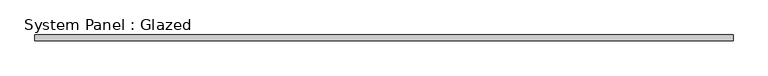
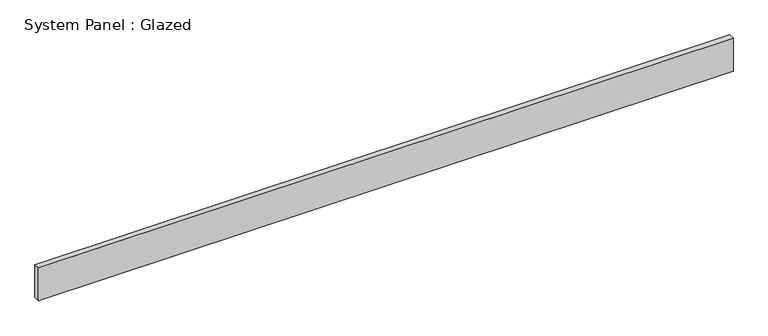
"""IFC4 building model written with IfcOpenShell, lengths in millimetres: plate geometry, System Panel : Glazed."""

from ifc_helpers import new_model, si_unit, origin, origin_with_axes, place, context, project, spatial, polyline, outline, extrude, source, transform, mapped, element, save


def system_panel_glazed_48f0744a(model_context):
    return source(origin(), model_context, "Body", "SweptSolid", [
        extrude(outline(polyline([(1524.0, 19.05), (-1524.0, 19.05), (-1524.0, 44.45), (1524.0, 44.45), (1524.0, 19.05)])), origin_with_axes(), (0.0, 0.0, 1.0), 152.4),
    ])


if __name__ == "__main__":
    model = new_model("IFC4")
    model_context = context("Model", 3, world=origin())
    ifc_project = project(units=[si_unit("LENGTHUNIT", "METRE", prefix="MILLI")], contexts=[model_context])
    site = spatial("IfcSite", under=ifc_project)
    building = spatial("IfcBuilding", under=site)
    placement = place(None, origin())
    system_panel_glazed_shape = system_panel_glazed_48f0744a(model_context)
    element("IfcPlate", 1, ObjectType="System Panel : Glazed", at=placement, inside=building, context=model_context, shape_type="MappedRepresentation", body=[
        mapped(system_panel_glazed_shape, transform((0.0, 0.0, 0.0), x_axis=(1.0, 0.0, 0.0), y_axis=(0.0, 1.0, 0.0), z_axis=(0.0, 0.0, 1.0))),
    ])
    save(model, "model.ifc")

# Revit data of these elements
# Type "System Panel : Glazed"
#   Construction Type Id = "GSP4R"
#   Analytic Construction = "1/8 in Pilkington single glazing"
#   Visual Light Transmittance = 0.9
#   Solar Heat Gain Coefficient = 0.86
#   Heat Transfer Coefficient (U) = 1.18115 BTU/(h·ft²·°F)
#   Define Thermal Properties by = 1
# Element 1 (IfcPlate, "System Panel : Glazed")
#   Materials on its faces: "Glass"
# Materials
#   "Glass": class "Glass", colour RGB 0 128 192, transparency 0.75, Description = "Soda Lime Glass", Cost = 0
